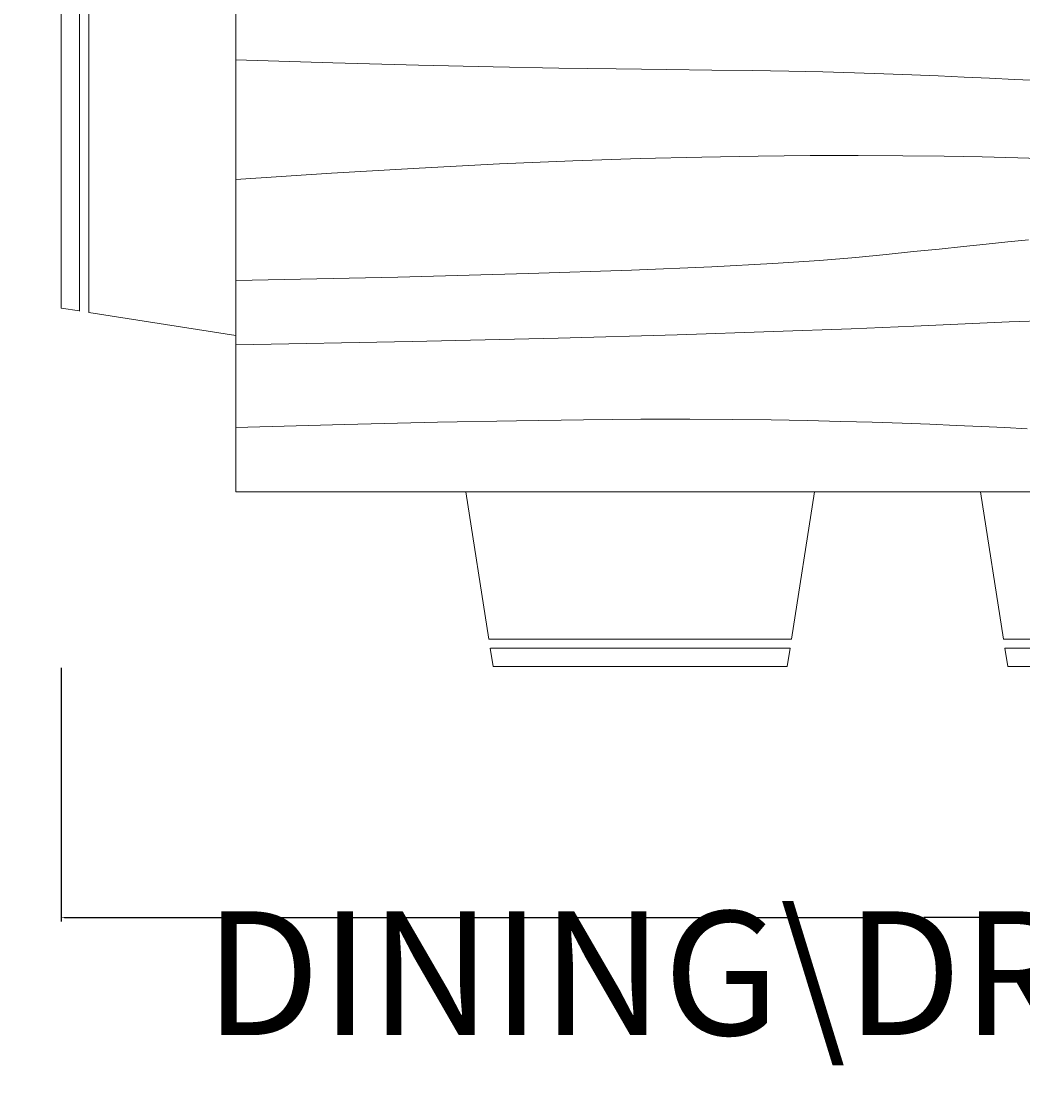
# Model space of a CAD drawing. Units: inches. Extents: x 4159 to 4826, y 299 to 1026.
# Tile 21 of 37: x 4305 to 4354, y 559 to 611. Entities that reach past the tile are written whole.
import ezdxf

# ---------------------------------------------------------------- set-up
doc = ezdxf.new("R2010")
doc.units = ezdxf.units.IN
for name, color, linetype, lineweight in [('A-ANNO-DIMS', 2, 'Continuous', 18), ('A-AREA-IDEN', 7, 'Continuous', 18), ('A-FURN', 8, 'Continuous', 18)]:
    doc.layers.add(name, color=color, linetype=linetype, lineweight=lineweight)
doc.styles.get("Standard").update_dxf_attribs({"font": 'arial.ttf'})
doc.dimstyles.get("Standard").update_dxf_attribs({"dimtxt": 0.18, "dimasz": 0.18, "dimexe": 0.18, "dimexo": 0.0625, "dimgap": 0.09, "dimtad": 0, "dimtih": 1, "dimtoh": 1, "dimdec": 4, "dimzin": 0, "dimdsep": 46, "dimtxsty": 'Standard', "dimcen": 0.09, "dimadec": 0, "dimazin": 0, "dimtfac": 1, "dimtdec": 4, "dimtofl": 0, "dimtmove": 0, "dimatfit": 3, "dimfxl": 1, "dimtolj": 1, "dimtzin": 0, "dimarcsym": 0})

# ---------------------------------------------------------------- blocks, each defined once
blk = doc.blocks.new('Dining Set - 36 x 72 in.')
for p, q in [((-36, 18), (-36, -18)), ((-44, 8.23041), (-44, -8.23915)), ((-45.5, 8), (-45.5, -8)), ((-44.5, -8.15843), (-44.5, 8.15338)), ((-44.4997, -8.15631), (-45.5, -8)), ((-35.9976, -9.48476), (-43.9993, -8.2345)), ((-36, -18), (36, -18)), ((-22.2343, -26.0006), (-23.4847, -17.99762)), ((-4.5152, -17.99762), (-5.7655, -25.99928)), ((5.7657, -26.0006), (4.5153, -17.99762)), ((-22.2304, -26), (-5.7608, -26)), ((5.7696, -26), (22.2392, -26)), ((-22, -27.5), (-22.1562, -26.50044)), ((-5.8416, -26.5), (-22.1534, -26.5)), ((-5.8437, -26.49967), (-6, -27.5)), ((6, -27.5), (5.8438, -26.50044)), ((22.1584, -26.5), (5.8466, -26.5)), ((-22, -27.5), (-6, -27.5)), ((6, -27.5), (22, -27.5))]:
    blk.add_line(p, q)
for points in [[(-36, 5.5), (-30.7157, 5.3348), (-26.069, 5.20963), (-21.9946, 5.11767), (-18.4271, 5.05208), (-15.3009, 5.00602), (-12.5508, 4.97265), (-10.1112, 4.94515), (-7.9167, 4.91666), (-5.909, 4.88167), (-4.0586, 4.83984), (-2.3429, 4.79215), (-0.7396, 4.73958), (0.7739, 4.6831), (2.22, 4.6237), (3.6213, 4.56233), (5, 4.5), (6.373, 4.43782), (7.7344, 4.3776)], [(-36, -1), (-30.7915, -0.6591), (-26.0195, -0.38216), (-21.6519, -0.16284), (-17.6563, 0.00521), (-14.0005, 0.12833), (-10.6523, 0.21289), (-7.5796, 0.26522), (-4.75, 0.29166), (-2.134, 0.29793), (0.2878, 0.28711), (2.5317, 0.26163), (4.6146, 0.22396), (6.5529, 0.17651), (8.3633, 0.12174)], [(-36, -6.5), (-27.1843, -6.31267), (-20.084, -6.1263), (-14.469, -5.9419), (-10.1094, -5.76042), (-6.7752, -5.58285), (-4.2363, -5.41016), (-2.2629, -5.24333), (-0.625, -5.08334), (0.8708, -4.93099), (2.2715, -4.78646), (3.5872, -4.64974), (4.8281, -4.52084), (6.0046, -4.39974), (7.127, -4.28646)], [(-36, -10), (-26.4022, -9.81299), (-18.4675, -9.62891), (-11.9839, -9.45069), (-6.7396, -9.28125), (-2.5226, -9.12354), (0.8789, -8.98047), (3.6769, -8.85498), (6.0833, -8.75), (8.2767, -8.66765)], [(-36, -14.5), (-30.0881, -14.33513), (-25.0332, -14.21224), (-20.7312, -14.12647), (-17.0781, -14.07292), (-13.97, -14.04671), (-11.3027, -14.04297), (-8.9724, -14.05681), (-6.875, -14.08334), (-4.9224, -14.11833), (-3.0905, -14.16016), (-1.3709, -14.20785), (0.2448, -14.26042), (1.7647, -14.3169), (3.1973, -14.3763), (4.5507, -14.43767), (5.8333, -14.5), (7.0554, -14.5621)]]:
    blk.add_lwpolyline(points)
blk = doc.blocks.new('*D35')
at = {"layer": 'A-ANNO-DIMS', "color": 0, "lineweight": -2, "transparency": 16777216}
for p, q in [((4307.16, 579.671), (4307.16, 567.387)), ((4388.274, 579.671), (4388.274, 567.387)), ((4307.34, 567.567), (4346.439, 567.567)), ((4388.094, 567.567), (4348.995, 567.567))]:
    blk.add_line(p, q, dxfattribs=at)
at = {"layer": 'A-ANNO-DIMS', "color": 0, "transparency": 16777216}
for points in [[(4307.34, 567.597), (4307.34, 567.537), (4307.16, 567.567)], [(4388.094, 567.597), (4388.094, 567.537), (4388.274, 567.567)]]:
    blk.add_solid(points, dxfattribs=at)
at = {"layer": 'Defpoints', "color": 0, "transparency": 16777216}
for p in [(4307.16, 579.734), (4388.274, 579.734), (4388.274, 567.567)]:
    blk.add_point(p, dxfattribs=at)
at = {"layer": 'A-ANNO-DIMS', "color": 0, "transparency": 16777216, "insert": (4347.717, 567.567), "char_height": 0.18, "attachment_point": 5}
blk.add_mtext('\\A1;DINING SET 81 TYP.', dxfattribs=at)
blk = doc.blocks.new('*D44')
at = {"layer": 'A-ANNO-DIMS', "color": 0, "lineweight": -2, "transparency": 16777216}
for p, q in [((4287.263, 963.093), (4158.88, 963.093)), ((4159.06, 962.913), (4159.06, 647.826)), ((4159.06, 332.375), (4159.06, 647.462)), ((4447.248, 332.195), (4158.88, 332.195))]:
    blk.add_line(p, q, dxfattribs=at)
at = {"layer": 'A-ANNO-DIMS', "color": 0, "transparency": 16777216}
for points in [[(4159.03, 962.913), (4159.09, 962.913), (4159.06, 963.093)], [(4159.03, 332.375), (4159.09, 332.375), (4159.06, 332.195)]]:
    blk.add_solid(points, dxfattribs=at)
at = {"layer": 'Defpoints', "color": 0, "transparency": 16777216}
for p in [(4287.326, 963.093), (4159.06, 332.195), (4447.31, 332.195)]:
    blk.add_point(p, dxfattribs=at)
at = {"layer": 'A-ANNO-DIMS', "color": 0, "transparency": 16777216, "insert": (4159.06, 647.644), "char_height": 0.18, "attachment_point": 5}
blk.add_mtext('\\A1;630.9', dxfattribs=at)

msp = doc.modelspace()

# ---------------------------------------------------------------- block references
at = {"layer": 'A-FURN', "xscale": 0.8913588978043845, "yscale": 0.8913588978043845, "zscale": 0.8913588978043845}
msp.add_blockref('Dining Set - 36 x 72 in.', (4347.717, 604.246), dxfattribs=at)

# ---------------------------------------------------------------- texts
at = {"layer": 'A-AREA-IDEN'}
msp.add_text('DINING\\DRAWING', height=6, dxfattribs=at).set_placement((4314.093, 561.874))

# ---------------------------------------------------------------- dimensions: what is measured, and where the dimension line sits
at = {"layer": 'A-ANNO-DIMS'}
dim = msp.add_linear_dim(base=(4159.06, 332.195), p1=(4287.326, 963.093), p2=(4447.31, 332.195), angle=90, dimstyle='Standard', override={"dimdec": 1, "dimlfac": 1, "dimrnd": 0, "dimzin": 0, "dimdsep": 46, "dimlunit": 2}, dxfattribs=at)
dim.commit()
dim.dimension.update_dxf_attribs({"geometry": '*D44', "text_midpoint": (4159.06, 647.644)})
dim = msp.add_linear_dim(base=(4388.274, 567.567), p1=(4307.16, 579.734), p2=(4388.274, 579.734), text='DINING SET <> TYP.', dimstyle='Standard', override={"dimdec": 0, "dimlfac": 1, "dimrnd": 0, "dimzin": 0, "dimdsep": 46, "dimlunit": 2}, dxfattribs=at)
dim.commit()
dim.dimension.update_dxf_attribs({"geometry": '*D35', "text_midpoint": (4347.717, 567.567)})

doc.saveas('drawing.dxf')
